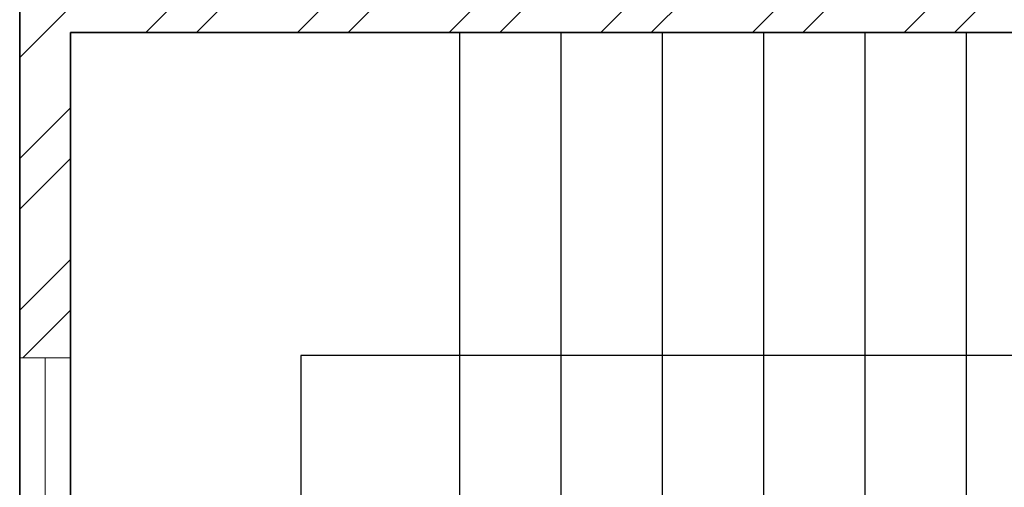
# Model space of a CAD drawing. Units: inches. Extents: x 1962 to 2771, y 1245 to 2660.
# Tile 35 of 114: x 2072 to 2159, y 1989 to 2030. Entities that reach past the tile are written whole.
import ezdxf

# ---------------------------------------------------------------- set-up
doc = ezdxf.new("R2010")
doc.units = ezdxf.units.IN
for name, color, linetype, lineweight in [('A-FLOR-STRS', 7, 'Continuous', 25), ('A-GLAZ', 4, 'Continuous', 18), ('A-WALL', 7, 'Continuous', 35), ('A-WALL-PATT', 252, 'Continuous', 13)]:
    doc.layers.add(name, color=color, linetype=linetype, lineweight=lineweight)

msp = doc.modelspace()

# ---------------------------------------------------------------- hatches: boundary and pattern name
at = {"layer": 'A-WALL-PATT'}
h = msp.add_hatch(dxfattribs=at)
h.set_pattern_fill('ANSI32', color=256)
h.paths.add_polyline_path([(2090.8074, 2467.3437), (2141.6481, 2467.3437), (2141.6481, 2469.5937), (2141.6481, 2471.8437), (2086.3074, 2471.8437), (2086.3074, 2422.5333), (2090.8074, 2422.5333)])
h.paths.add_polyline_path([(2282.7664, 2471.8437), (2204.8982, 2471.8437), (2204.8982, 2467.3437), (2234.8074, 2467.3437), (2234.8074, 2311.3437), (2228.7492, 2311.3437), (2228.7492, 2306.8437), (2234.8074, 2306.8437), (2331.9227, 2306.8437), (2331.9227, 2309.0937), (2331.9227, 2311.3437), (2239.3074, 2311.3437), (2239.3074, 2467.3437), (2282.7664, 2467.3437), (2282.7664, 2469.5937)])
h.paths.add_polyline_path([(2471.4531, 2519.8437), (2552.011, 2519.8437), (2564.3996, 2519.8437), (2564.3996, 2511.1389), (2568.8996, 2511.1389), (2568.8996, 2524.3437), (2466.9531, 2524.3437), (2466.9531, 2471.8437), (2450.0749, 2471.8437), (2446.4672, 2471.8437), (2446.4672, 2467.3437), (2450.0749, 2467.3437), (2475.9988, 2467.3437), (2475.9988, 2469.5937), (2475.9988, 2471.8437), (2471.4531, 2471.8437)])
h.paths.add_polyline_path([(2575.2231, 2469.5937), (2575.2231, 2471.8437), (2568.8996, 2471.8437), (2568.8996, 2487.1389), (2564.3996, 2487.1389), (2564.3996, 2471.8437), (2556.511, 2471.8437), (2499.2904, 2471.8437), (2499.2904, 2467.3437), (2507.8074, 2467.3437), (2507.8074, 2311.3437), (2414.863, 2311.3437), (2414.863, 2306.8437), (2512.3074, 2306.8437), (2517.0114, 2306.8437), (2517.0114, 2309.0937), (2517.0114, 2311.3437), (2512.3074, 2311.3437), (2512.3074, 2467.3437), (2575.2231, 2467.3437)])
h.paths.add_polyline_path([(2660.8074, 2471.8437), (2600.9602, 2471.8437), (2600.9602, 2467.3437), (2656.3074, 2467.3437), (2656.3074, 2432.5704), (2660.8074, 2432.5704)])
h.paths.add_polyline_path([(2660.8074, 2372.5704), (2656.3074, 2372.5704), (2656.3074, 2311.3437), (2600.276, 2311.3437), (2600.276, 2309.0937), (2600.276, 2306.8437), (2656.3074, 2306.8437), (2656.3074, 2296.2593), (2660.8074, 2296.2593)])
h.paths.add_polyline_path([(2572.3074, 2306.8437), (2577.1385, 2306.8437), (2577.1385, 2311.3437), (2551.082, 2311.3437), (2551.082, 2306.8437), (2567.8074, 2306.8437), (2567.8074, 2258.8437), (2540.0574, 2258.8437), (2540.0574, 2256.5937), (2540.0574, 2254.3437), (2567.8074, 2254.3437), (2656.3074, 2254.3437), (2656.3074, 2236.9085), (2660.8074, 2236.9085), (2660.8074, 2272.2593), (2656.3074, 2272.2593), (2656.3074, 2258.8437), (2572.3074, 2258.8437)])
h.paths.add_polyline_path([(2512.3074, 2254.3437), (2518.8716, 2254.3437), (2518.8716, 2256.5937), (2518.8716, 2258.8437), (2507.8074, 2258.8437), (2507.8074, 2177.8437), (2567.8074, 2177.8437), (2567.8074, 2172.9628), (2572.3074, 2172.9628), (2572.3074, 2177.8437), (2656.3074, 2177.8437), (2656.3074, 2166.4846), (2660.8074, 2166.4846), (2660.8074, 2200.9085), (2656.3074, 2200.9085), (2656.3074, 2182.3437), (2512.3074, 2182.3437)])
h.paths.add_polyline_path([(2656.3074, 2129.8437), (2572.3074, 2129.8437), (2572.3074, 2150.3044), (2570.0574, 2150.3044), (2567.8074, 2150.3044), (2567.8074, 2129.8437), (2507.8074, 2129.8437), (2507.8074, 2116.3027), (2510.0574, 2116.3027), (2512.3074, 2116.3027), (2512.3074, 2125.3437), (2567.8074, 2125.3437), (2572.3074, 2125.3437), (2656.3074, 2125.3437)])
h.paths.add_polyline_path([(2090.8074, 2362.5333), (2086.3074, 2362.5333), (2086.3074, 2298.6242), (2090.8074, 2298.6242), (2090.8074, 2306.8437), (2174.8074, 2306.8437), (2174.8074, 2286.4178), (2179.3074, 2286.4178), (2179.3074, 2306.8437), (2192.8641, 2306.8437), (2192.8641, 2309.0937), (2192.8641, 2311.3437), (2090.8074, 2311.3437)])
h.paths.add_polyline_path([(2209.156, 2258.8437), (2179.3074, 2258.8437), (2179.3074, 2263.2236), (2177.0574, 2263.2236), (2174.8074, 2263.2236), (2174.8074, 2258.8437), (2090.8074, 2258.8437), (2090.8074, 2274.6242), (2086.3074, 2274.6242), (2086.3074, 2238.2967), (2088.5574, 2238.2967), (2090.8074, 2238.2967), (2090.8074, 2254.3437), (2209.156, 2254.3437)])
h.paths.add_polyline_path([(2090.8074, 2177.8437), (2234.8074, 2177.8437), (2234.8074, 2173.1428), (2239.3074, 2173.1428), (2239.3074, 2258.8437), (2230.8442, 2258.8437), (2230.8442, 2256.5937), (2230.8442, 2254.3437), (2234.8074, 2254.3437), (2234.8074, 2182.3437), (2090.8074, 2182.3437), (2090.8074, 2202.2967), (2086.3074, 2202.2967), (2086.3074, 2140.0389), (2090.8074, 2140.0389)])
h.paths.add_polyline_path([(2090.8074, 2080.0389), (2086.3074, 2080.0389), (2086.3074, 2033.8437), (2090.8074, 2033.8437)], flags=17)
h.paths.add_polyline_path([(2244.9405, 2033.8437), (2239.3074, 2033.8437), (2239.3074, 2142.0665), (2237.2592, 2142.0665), (2234.8074, 2142.0665), (2234.8074, 2033.8437), (2090.8074, 2033.8437), (2076.5204, 2033.8437), (2072.0204, 2033.8437), (2072.0204, 2000.4493), (2076.5204, 2000.4493), (2076.5204, 2029.3437), (2090.8074, 2029.3437), (2244.9405, 2029.3437), (2244.9405, 2031.5937)])
h.paths.add_polyline_path([(2234.8074, 1933.3437), (2076.5204, 1933.3437), (2076.5204, 1952.4493), (2074.2704, 1952.4493), (2072.0204, 1952.4493), (2072.0204, 1933.3437), (2072.0204, 1928.8437), (2234.8074, 1928.8437)])
h.paths.add_polyline_path([(2090.8074, 1928.8437), (2086.3074, 1928.8437), (2086.3074, 1906.5013), (2090.8074, 1906.5013)])
h.paths.add_polyline_path([(2090.8074, 1846.5013), (2086.3074, 1846.5013), (2086.3074, 1769.9917), (2088.5574, 1769.9917), (2090.8074, 1769.9917), (2090.8074, 1780.3437), (2234.8074, 1780.3437), (2234.8074, 1708.3437), (2230.3764, 1708.3437), (2230.3764, 1703.8437), (2239.3074, 1703.8437), (2239.3074, 1792.6669), (2237.0574, 1792.6669), (2234.8074, 1792.6669), (2234.8074, 1784.8437), (2090.8074, 1784.8437)])
h.paths.add_polyline_path([(2239.3074, 1928.8437), (2244.9405, 1928.8437), (2244.9405, 1931.0937), (2244.9405, 1933.3437), (2234.8074, 1933.3437), (2234.8074, 1928.8437), (2234.8074, 1825.5949), (2239.3074, 1825.5949)])
h.paths.add_polyline_path([(2148.0425, 1649.0937), (2148.0425, 1651.3437), (2090.8074, 1651.3437), (2090.8074, 1646.8437), (2148.0425, 1646.8437)], flags=0)
h.paths.add_polyline_path([(2207.5601, 1708.3437), (2090.8074, 1708.3437), (2090.8074, 1703.8437), (2174.8074, 1703.8437), (2174.8074, 1651.3437), (2170.4457, 1651.3437), (2170.4457, 1646.8437), (2195.9924, 1646.8437), (2195.9924, 1649.0937), (2195.9924, 1651.3437), (2179.3074, 1651.3437), (2179.3074, 1703.8437), (2207.5601, 1703.8437), (2207.5601, 1706.0937)])
h.paths.add_polyline_path([(2090.8074, 1733.9917), (2086.3074, 1733.9917), (2086.3074, 1696.1032), (2088.5574, 1696.1032), (2090.8074, 1696.1032)])
h.paths.add_polyline_path([(2090.8074, 1672.1032), (2086.3074, 1672.1032), (2086.3074, 1600.3335), (2090.8074, 1600.3335)])
h.paths.add_polyline_path([(2090.8074, 1540.3335), (2086.3074, 1540.3335), (2086.3074, 1486.3437), (2139.6766, 1486.3437), (2139.6766, 1490.8437), (2090.8074, 1490.8437)])
h.paths.add_polyline_path([(2302.3876, 1490.8437), (2239.3074, 1490.8437), (2239.3074, 1646.8437), (2335.9994, 1646.8437), (2335.9994, 1651.3437), (2229.884, 1651.3437), (2229.884, 1646.8437), (2234.8074, 1646.8437), (2234.8074, 1490.8437), (2202.7103, 1490.8437), (2202.7103, 1488.5937), (2202.7103, 1486.3437), (2275.0699, 1486.3437), (2275.0699, 1475.772), (2279.5699, 1475.772), (2279.5699, 1486.3437), (2302.3876, 1486.3437)])
h.paths.add_polyline_path([(2279.5699, 1451.772), (2275.0699, 1451.772), (2275.0699, 1438.3437), (2174.8074, 1438.3437), (2174.8074, 1486.3437), (2179.7922, 1486.3437), (2179.7922, 1490.8437), (2163.3585, 1490.8437), (2163.3585, 1488.5937), (2163.3585, 1486.3437), (2170.3074, 1486.3437), (2170.3074, 1433.8437), (2279.5699, 1433.8437)])
h.paths.add_polyline_path([(2427.2363, 1490.8437), (2375.8074, 1490.8437), (2375.8074, 1646.8437), (2381.6401, 1646.8437), (2381.6401, 1651.3437), (2365.887, 1651.3437), (2365.887, 1649.0937), (2365.887, 1646.8437), (2371.3074, 1646.8437), (2371.3074, 1490.8437), (2327.5627, 1490.8437), (2327.5627, 1488.5937), (2327.5627, 1486.3437), (2371.3074, 1486.3437), (2371.3074, 1433.8437), (2375.8074, 1433.8437), (2375.8074, 1486.3437), (2427.2363, 1486.3437)])
h.paths.add_polyline_path([(2512.3074, 1646.8437), (2519.4351, 1646.8437), (2519.4351, 1649.0937), (2519.4351, 1651.3437), (2507.8074, 1651.3437), (2416.0063, 1651.3437), (2416.0063, 1649.0937), (2416.0063, 1646.8437), (2507.8074, 1646.8437), (2507.8074, 1490.8437), (2497.0532, 1490.8437), (2497.0532, 1488.5937), (2497.0532, 1486.3437), (2574.9344, 1486.3437), (2574.9344, 1476.0181), (2579.4344, 1476.0181), (2579.4344, 1486.3437), (2584.4872, 1486.3437), (2584.3074, 1490.8437), (2512.3074, 1490.8437)])
h.paths.add_polyline_path([(2470.5091, 1486.3437), (2473.9767, 1486.3437), (2473.9767, 1490.8437), (2449.6605, 1490.8437), (2449.6605, 1488.5937), (2449.6605, 1486.3437), (2466.0091, 1486.3437), (2466.0091, 1433.8437), (2470.5091, 1433.8437), (2579.4344, 1433.8437), (2579.4344, 1452.0181), (2574.9344, 1452.0181), (2574.9344, 1438.3437), (2554.5091, 1438.3437), (2470.5091, 1438.3437)])
h.paths.add_polyline_path([(2656.3074, 1490.8437), (2611.86, 1490.8437), (2611.86, 1486.3437), (2656.3074, 1486.3437)])
h.paths.add_polyline_path([(2660.8074, 1532.7007), (2658.5574, 1532.7007), (2656.3074, 1532.7007), (2656.3074, 1486.3437), (2660.8074, 1486.3437)])
h.paths.add_polyline_path([(2660.8074, 1664.9663), (2656.3074, 1664.9663), (2656.3074, 1651.3437), (2602.2313, 1651.3437), (2602.2313, 1646.8437), (2656.3074, 1646.8437), (2656.3074, 1592.7007), (2660.8074, 1592.7007)])
h.paths.add_polyline_path([(2660.8074, 1724.5221), (2656.3074, 1724.5221), (2656.3074, 1703.8437), (2542.4725, 1703.8437), (2542.4725, 1699.3437), (2567.8074, 1699.3437), (2567.8074, 1651.3437), (2552.7766, 1651.3437), (2552.7766, 1649.0937), (2552.7766, 1646.8437), (2577.2878, 1646.8437), (2577.2878, 1649.0937), (2577.2878, 1651.3437), (2572.3074, 1651.3437), (2572.3074, 1699.3437), (2656.3074, 1699.3437), (2656.3074, 1688.9663), (2660.8074, 1688.9663)])
h.paths.add_polyline_path([(2660.8074, 1880.6524), (2656.3074, 1880.6524), (2656.3074, 1832.8437), (2512.3074, 1832.8437), (2512.3074, 1837.8959), (2507.8074, 1837.8959), (2507.8074, 1828.3437), (2567.8074, 1828.3437), (2567.8074, 1804.3437), (2572.3074, 1804.3437), (2572.3074, 1828.3437), (2656.3074, 1828.3437), (2656.3074, 1818.6778), (2660.8074, 1818.6778)])
h.paths.add_polyline_path([(2660.8074, 1794.6778), (2656.3074, 1794.6778), (2656.3074, 1780.3437), (2572.3074, 1780.3437), (2572.3074, 1783.0303), (2570.0574, 1783.0303), (2567.8074, 1783.0303), (2567.8074, 1780.3437), (2507.8074, 1780.3437), (2507.8074, 1699.3437), (2517.8858, 1699.3437), (2517.8858, 1701.5937), (2517.8858, 1703.8437), (2512.3074, 1703.8437), (2512.3074, 1775.8437), (2656.3074, 1775.8437), (2656.3074, 1760.5221), (2660.8074, 1760.5221)])
h.paths.add_polyline_path([(2660.8074, 1981.3437), (2660.8074, 2020.2808), (2658.5574, 2020.2808), (2656.3074, 2020.2808), (2656.3074, 1981.3437), (2512.3074, 1981.3437), (2512.3074, 2086.6996), (2507.8074, 2086.6996), (2507.8074, 1981.3437), (2375.8074, 1981.3437), (2375.8074, 1986.8505), (2373.5574, 1986.8505), (2371.3074, 1986.8505), (2371.3074, 1973.2607), (2375.8074, 1973.2607), (2375.8074, 1976.8437), (2507.8074, 1976.8437), (2507.8074, 1865.4281), (2510.0574, 1865.4281), (2512.3074, 1865.4281), (2512.3074, 1976.8437), (2660.8074, 1976.8437)])
h.paths.add_polyline_path([(2375.8074, 1940.297), (2373.5574, 1940.297), (2371.3074, 1940.297), (2371.3074, 1933.3437), (2278.4434, 1933.3437), (2278.4434, 1928.8437), (2371.3074, 1928.8437), (2371.3074, 1651.3437), (2375.8074, 1651.3437)])
h.paths.add_polyline_path([(2660.8074, 1976.8437), (2656.3074, 1976.8437), (2656.3074, 1940.6524), (2660.8074, 1940.6524)], flags=17)
h.paths.add_polyline_path([(2660.8074, 2142.4846), (2656.3074, 2142.4846), (2656.3074, 2080.2808), (2660.8074, 2080.2808)])
h.paths.add_polyline_path([(2381.4189, 2311.3437), (2375.8074, 2311.3437), (2375.8074, 2467.3437), (2424.7242, 2467.3437), (2424.7242, 2469.5937), (2424.7242, 2471.8437), (2375.8074, 2471.8437), (2375.8074, 2524.3437), (2371.3074, 2524.3437), (2371.3074, 2471.8437), (2307.2097, 2471.8437), (2307.2097, 2467.3437), (2371.3074, 2467.3437), (2371.3074, 2311.3437), (2366.8901, 2311.3437), (2366.8901, 2306.8437), (2371.3074, 2306.8437), (2371.3074, 2033.8437), (2279.6589, 2033.8437), (2279.6589, 2029.3437), (2371.3074, 2029.3437), (2371.3074, 2014.2598), (2375.8074, 2014.2598), (2375.8074, 2306.8437), (2381.4189, 2306.8437)])
h.paths.add_polyline_path([(2263.3074, 2524.3437), (2170.3074, 2524.3437), (2170.3074, 2519.8437), (2170.3074, 2471.8437), (2165.0312, 2471.8437), (2165.0312, 2467.3437), (2179.6721, 2467.3437), (2179.6721, 2469.5161), (2179.6721, 2471.8437), (2174.8074, 2471.8437), (2174.8074, 2519.8437), (2258.8074, 2519.8437), (2258.8074, 2511.6436), (2263.3074, 2511.6436)])
h.paths.add_polyline_path([(2245.0232, 1361.4123), (2492.9468, 1361.4123), (2492.9468, 1398.505), (2245.0232, 1398.505)], flags=9)
h.paths.add_polyline_path([(2388.1434, 2086.6936), (2425.0704, 2086.6936), (2425.0704, 2105.3509), (2388.1434, 2105.3509)], flags=9)
h.paths.add_polyline_path([(2404.922, 2242.6744), (2445.7337, 2242.6744), (2445.7337, 2261.3318), (2404.922, 2261.3318)], flags=9)
h.paths.add_polyline_path([(2269.4107, 2156.7935), (2306.3378, 2156.7935), (2306.3378, 2175.4508), (2269.4107, 2175.4508)], flags=9)
h.paths.add_polyline_path([(2269.3277, 2233.4343), (2306.2547, 2233.4343), (2306.2547, 2252.0917), (2269.3277, 2252.0917)], flags=9)
h.paths.add_polyline_path([(2431.6052, 2320.6922), (2470.4456, 2320.6922), (2470.4456, 2339.3495), (2431.6052, 2339.3495)], flags=25)
h.paths.add_polyline_path([(2249.6902, 2315.7608), (2288.5306, 2315.7608), (2288.5306, 2334.4182), (2249.6902, 2334.4182)], flags=25)
h.paths.add_polyline_path([(2096.9301, 2314.3181), (2135.7704, 2314.3181), (2135.7704, 2332.9755), (2096.9301, 2332.9755)], flags=25)
h.paths.add_polyline_path([(2134.3475, 2285.7089), (2161.4655, 2285.7089), (2161.4655, 2304.3662), (2134.3475, 2304.3662)], flags=9)
h.paths.add_polyline_path([(2126.5155, 2209.4076), (2159.9227, 2209.4076), (2159.9227, 2228.065), (2126.5155, 2228.065)], flags=25)
h.paths.add_polyline_path([(2110.5753, 2141.5299), (2149.4157, 2141.5299), (2149.4157, 2160.1872), (2110.5753, 2160.1872)], flags=25)
h.paths.add_polyline_path([(2249.8618, 1968.3317), (2286.3966, 1968.3317), (2286.3966, 1986.989), (2249.8618, 1986.989)], flags=9)
h.paths.add_polyline_path([(2395.9507, 1777.0051), (2436.7624, 1777.0051), (2436.7624, 1795.6625), (2395.9507, 1795.6625)], flags=9)
h.paths.add_polyline_path([(2398.5259, 1888.5651), (2435.0062, 1888.5651), (2435.0062, 1907.2224), (2398.5259, 1907.2224)], flags=25)
h.paths.add_polyline_path([(2259.3506, 1728.3559), (2296.2776, 1728.3559), (2296.2776, 1747.0132), (2259.3506, 1747.0132)], flags=9)
h.paths.add_polyline_path([(2271.3698, 1845.268), (2308.2968, 1845.268), (2308.2968, 1863.9253), (2271.3698, 1863.9253)], flags=9)
h.paths.add_polyline_path([(2120.9355, 1786.3027), (2159.7759, 1786.3027), (2159.7759, 1804.9601), (2120.9355, 1804.9601)], flags=25)
h.paths.add_polyline_path([(2121.3164, 1732.1043), (2154.7236, 1732.1043), (2154.7236, 1750.7616), (2121.3164, 1750.7616)], flags=25)
h.paths.add_polyline_path([(2118.3706, 1678.8997), (2147.5282, 1678.8997), (2147.5282, 1697.557), (2118.3706, 1697.557)], flags=25)
h.paths.add_polyline_path([(2385.9227, 1493.557), (2424.763, 1493.557), (2424.763, 1512.2143), (2385.9227, 1512.2143)], flags=25)
h.paths.add_polyline_path([(2248.7058, 1500.0256), (2287.5462, 1500.0256), (2287.5462, 1518.6829), (2248.7058, 1518.6829)], flags=25)
h.paths.add_polyline_path([(2104.1669, 1617.3771), (2143.0073, 1617.3771), (2143.0073, 1636.0344), (2104.1669, 1636.0344)], flags=9)
h.paths.add_polyline_path([(2096.0714, 1447.8824), (2137.3845, 1447.8824), (2137.3845, 1458.1859), (2096.0714, 1458.1859)], flags=9)
h.paths.add_polyline_path([(2180.6114, 1440.325), (2209.7689, 1440.325), (2209.7689, 1458.9823), (2180.6114, 1458.9823)], flags=25)
h.paths.add_polyline_path([(2316.1698, 1447.9637), (2357.4829, 1447.9637), (2357.4829, 1458.2673), (2316.1698, 1458.2673)], flags=9)
h.paths.add_polyline_path([(2397.6187, 1447.9637), (2438.9318, 1447.9637), (2438.9318, 1458.2673), (2397.6187, 1458.2673)], flags=9)
h.paths.add_polyline_path([(2473.0778, 1439.5953), (2502.2354, 1439.5953), (2502.2354, 1458.2527), (2473.0778, 1458.2527)], flags=25)
h.paths.add_polyline_path([(2589.7027, 1447.8819), (2631.0158, 1447.8819), (2631.0158, 1458.1855), (2589.7027, 1458.1855)], flags=9)
h.paths.add_polyline_path([(2522.4009, 1497.5285), (2561.2413, 1497.5285), (2561.2413, 1516.1859), (2522.4009, 1516.1859)], flags=25)
h.paths.add_polyline_path([(2579.6565, 1671.3482), (2608.8141, 1671.3482), (2608.8141, 1690.0056), (2579.6565, 1690.0056)], flags=25)
h.paths.add_polyline_path([(2544.7038, 1725.5064), (2578.1111, 1725.5064), (2578.1111, 1744.1637), (2544.7038, 1744.1637)], flags=25)
h.paths.add_polyline_path([(2578.1191, 1807.472), (2607.2766, 1807.472), (2607.2766, 1826.1293), (2578.1191, 1826.1293)], flags=25)
h.paths.add_polyline_path([(2595.0614, 1835.1839), (2633.9018, 1835.1839), (2633.9018, 1853.8413), (2595.0614, 1853.8413)], flags=25)
h.paths.add_polyline_path([(2567.0097, 2097.7035), (2605.8501, 2097.7035), (2605.8501, 2116.3609), (2567.0097, 2116.3609)], flags=9)
h.paths.add_polyline_path([(2586.644, 2134.6454), (2615.8015, 2134.6454), (2615.8015, 2153.3027), (2586.644, 2153.3027)], flags=9)
h.paths.add_polyline_path([(2544.6185, 2212.6783), (2578.0258, 2212.6783), (2578.0258, 2231.3356), (2544.6185, 2231.3356)], flags=25)
h.paths.add_polyline_path([(2577.0273, 2256.9023), (2606.1849, 2256.9023), (2606.1849, 2275.5597), (2577.0273, 2275.5597)], flags=24)
h.paths.add_polyline_path([(2605.2683, 2315.2821), (2644.1087, 2315.2821), (2644.1087, 2333.9395), (2605.2683, 2333.9395)], flags=25)
h.paths.add_polyline_path([(2583.1244, 2496.1815), (2624.4375, 2496.1815), (2624.4375, 2506.4851), (2583.1244, 2506.4851)], flags=9)
h.paths.add_polyline_path([(2474.761, 2497.0823), (2503.9185, 2497.0823), (2503.9185, 2515.7397), (2474.761, 2515.7397)], flags=25)
h.paths.add_polyline_path([(2387.5787, 2494.2563), (2428.902, 2494.2563), (2428.902, 2504.5598), (2387.5787, 2504.5598)], flags=9)
h.paths.add_polyline_path([(2300.1657, 2500.1564), (2341.4788, 2500.1564), (2341.4788, 2510.46), (2300.1657, 2510.46)], flags=25)
h.paths.add_polyline_path([(2176.8589, 2497.5843), (2206.0165, 2497.5843), (2206.0165, 2516.2416), (2176.8589, 2516.2416)], flags=25)
h.paths.add_polyline_path([(2097.4668, 2494.9762), (2138.7799, 2494.9762), (2138.7799, 2505.2798), (2097.4668, 2505.2798)], flags=9)

# ---------------------------------------------------------------- linework, layer by layer
at = {"layer": 'A-FLOR-STRS'}
for p, q in [((2111.0955, 2029.3437), (2111.0955, 1933.3437)), ((2120.0955, 2029.3437), (2120.0955, 1933.3437)), ((2129.0955, 2029.3437), (2129.0955, 1933.3437)), ((2138.0955, 2029.3437), (2138.0955, 1933.3437)), ((2147.0955, 2029.3437), (2147.0955, 1933.3437)), ((2156.0955, 2029.3437), (2156.0955, 1933.3437)), ((2242.2648, 2000.646), (2096.9843, 2000.646)), ((2096.9843, 2000.646), (2096.9843, 1948.6514))]:
    msp.add_line(p, q, dxfattribs=at)
at = {"layer": 'A-GLAZ'}
for p, q in [((2074.2704, 2000.4493), (2072.0204, 2000.4493)), ((2072.0204, 2000.4493), (2076.5204, 2000.4493)), ((2074.2704, 1952.4493), (2074.2704, 2000.4493))]:
    msp.add_line(p, q, dxfattribs=at)
at = {"layer": 'A-WALL'}
for p, q in [((2072.0204, 2033.8437), (2072.0204, 1933.3437)), ((2090.8074, 2029.3437), (2076.5204, 2029.3437)), ((2076.5204, 2029.3437), (2076.5204, 1933.3437)), ((2090.8074, 2029.3437), (2244.9405, 2029.3437))]:
    msp.add_line(p, q, dxfattribs=at)

doc.saveas('drawing.dxf')
